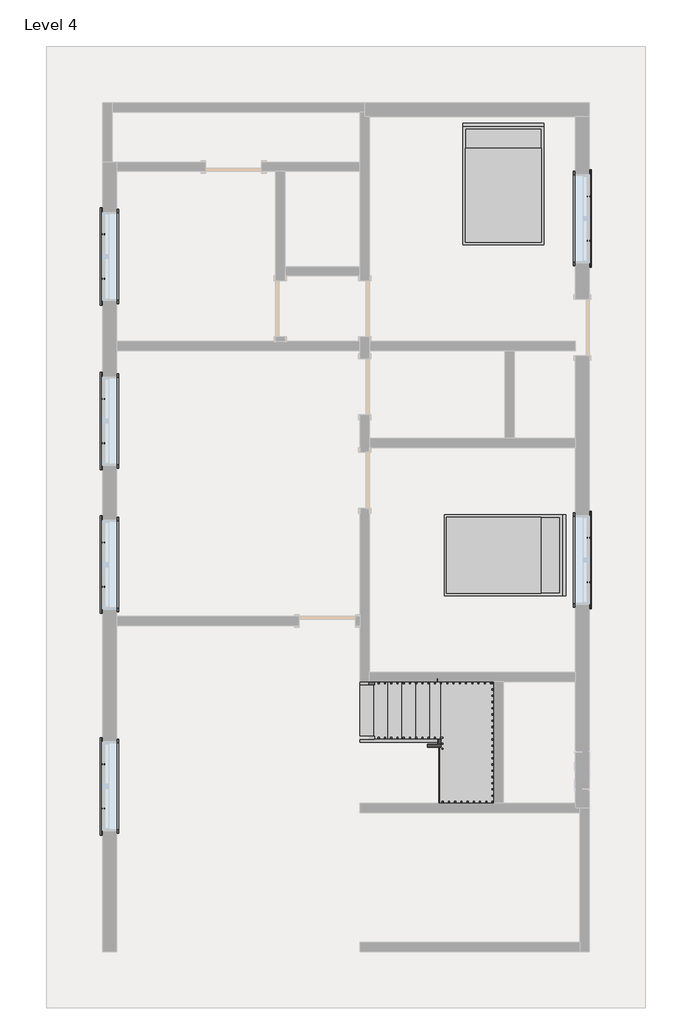
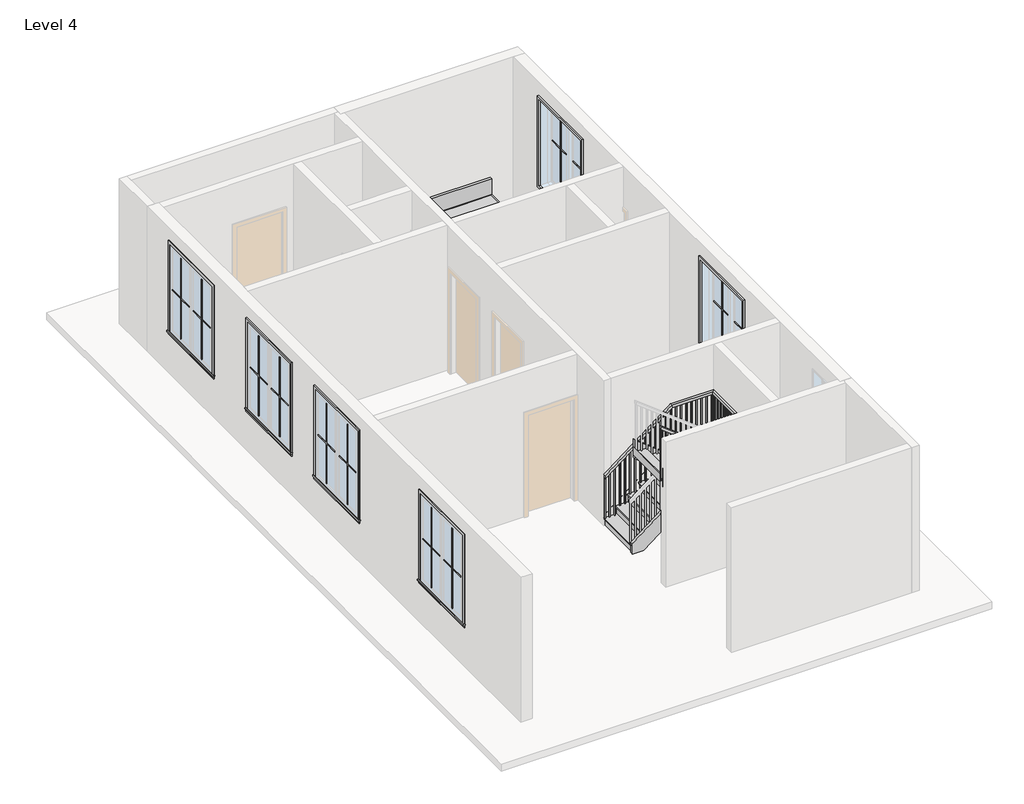
# One storey, part 2 of 2: 24 proxies, 6 members, 2 furniture elements, 1 railing, 1 stair flight.
"""IFC4 building model written with IfcOpenShell, lengths in millimetres."""

from ifc_helpers import new_model, si_unit, frame, origin, place, context, project, spatial, polyline, outline, extrude, faceted_brep, transform, mapped, element, save
from components import muntin_pattern_2x2_muntin_pattern_2x2_bff912c5, muntin_pattern_2x2_muntin_pattern_2x2_c2194282, trim_window_exterior_flat_with_sill_e04b3088, trim_window_interior_flat_picture_frame_2a7685fe, bed_17739_bed_17739_15c61121, stair_flight_6f98f22d

model = new_model("IFC4")

# Units and contexts
model_context = context("Model", 3, world=origin())
ifc_project = project(units=[si_unit("LENGTHUNIT", "METRE", prefix="MILLI")], contexts=[model_context])

# Site, building, storey
site = spatial("IfcSite", under=ifc_project)
building = spatial("IfcBuilding", under=site)
storey = spatial("IfcBuildingStorey", under=building, Name="Level 4", Elevation=6400.8)

# Proxies
placement = place(None, origin())
muntin_pattern_2x2_muntin_pattern_2x2_shape = muntin_pattern_2x2_muntin_pattern_2x2_bff912c5(model_context)
element("IfcBuildingElementProxy", 1, Name="Muntin Pattern_2x2 : Muntin Pattern_2x2", ObjectType="Muntin Pattern_2x2 : Muntin Pattern_2x2", at=placement, inside=storey, context=model_context, shape_type="MappedRepresentation", body=[
    mapped(muntin_pattern_2x2_muntin_pattern_2x2_shape, transform((-5204.1165352, 3633.8812696, 7385.05), x_axis=(0.0, 1.0, 0.0), y_axis=(-1.0, 0.0, 0.0), z_axis=(0.0, 0.0, 1.0))),
])
element("IfcBuildingElementProxy", 2, Name="Muntin Pattern_2x2 : Muntin Pattern_2x2", ObjectType="Muntin Pattern_2x2 : Muntin Pattern_2x2", at=placement, inside=storey, context=model_context, shape_type="MappedRepresentation", body=[
    mapped(muntin_pattern_2x2_muntin_pattern_2x2_shape, transform((2701.6334648, 4971.3355313, 7385.05), x_axis=(0.0, -1.0, 0.0), y_axis=(1.0, 0.0, 0.0), z_axis=(0.0, 0.0, 1.0))),
])
element("IfcBuildingElementProxy", 3, Name="Muntin Pattern_2x2 : Muntin Pattern_2x2", ObjectType="Muntin Pattern_2x2 : Muntin Pattern_2x2", at=placement, inside=storey, context=model_context, shape_type="MappedRepresentation", body=[
    mapped(muntin_pattern_2x2_muntin_pattern_2x2_shape, transform((2701.6334648, -584.9144687, 7385.05), x_axis=(0.0, -1.0, 0.0), y_axis=(1.0, 0.0, 0.0), z_axis=(0.0, 0.0, 1.0))),
])
element("IfcBuildingElementProxy", 4, Name="Muntin Pattern_2x2 : Muntin Pattern_2x2", ObjectType="Muntin Pattern_2x2 : Muntin Pattern_2x2", at=placement, inside=storey, context=model_context, shape_type="MappedRepresentation", body=[
    mapped(muntin_pattern_2x2_muntin_pattern_2x2_shape, transform((-5204.1165352, 954.9605313, 7385.05), x_axis=(0.0, 1.0, 0.0), y_axis=(-1.0, 0.0, 0.0), z_axis=(0.0, 0.0, 1.0))),
])
element("IfcBuildingElementProxy", 5, Name="Muntin Pattern_2x2 : Muntin Pattern_2x2", ObjectType="Muntin Pattern_2x2 : Muntin Pattern_2x2", at=placement, inside=storey, context=model_context, shape_type="MappedRepresentation", body=[
    mapped(muntin_pattern_2x2_muntin_pattern_2x2_shape, transform((-5204.1165352, -1381.8394687, 7385.05), x_axis=(0.0, 1.0, 0.0), y_axis=(-1.0, 0.0, 0.0), z_axis=(0.0, 0.0, 1.0))),
])
element("IfcBuildingElementProxy", 6, Name="Muntin Pattern_2x2 : Muntin Pattern_2x2", ObjectType="Muntin Pattern_2x2 : Muntin Pattern_2x2", at=placement, inside=storey, context=model_context, shape_type="MappedRepresentation", body=[
    mapped(muntin_pattern_2x2_muntin_pattern_2x2_shape, transform((-5204.1165352, -4988.6394687, 7385.05), x_axis=(0.0, 1.0, 0.0), y_axis=(-1.0, 0.0, 0.0), z_axis=(0.0, 0.0, 1.0))),
])
muntin_pattern_2x2_muntin_pattern_2x2_2_shape = muntin_pattern_2x2_muntin_pattern_2x2_c2194282(model_context)
element("IfcBuildingElementProxy", 7, Name="Muntin Pattern_2x2 : Muntin Pattern_2x2", ObjectType="Muntin Pattern_2x2 : Muntin Pattern_2x2", at=placement, inside=storey, context=model_context, shape_type="MappedRepresentation", body=[
    mapped(muntin_pattern_2x2_muntin_pattern_2x2_2_shape, transform((-5204.1165352, 4354.6062696, 7385.05), x_axis=(0.0, -1.0, 0.0), y_axis=(1.0, 0.0, 0.0), z_axis=(0.0, 0.0, 1.0))),
])
element("IfcBuildingElementProxy", 8, Name="Muntin Pattern_2x2 : Muntin Pattern_2x2", ObjectType="Muntin Pattern_2x2 : Muntin Pattern_2x2", at=placement, inside=storey, context=model_context, shape_type="MappedRepresentation", body=[
    mapped(muntin_pattern_2x2_muntin_pattern_2x2_2_shape, transform((2701.6334648, 4250.6105313, 7385.05), x_axis=(0.0, 1.0, 0.0), y_axis=(-1.0, 0.0, 0.0), z_axis=(0.0, 0.0, 1.0))),
])
element("IfcBuildingElementProxy", 9, Name="Muntin Pattern_2x2 : Muntin Pattern_2x2", ObjectType="Muntin Pattern_2x2 : Muntin Pattern_2x2", at=placement, inside=storey, context=model_context, shape_type="MappedRepresentation", body=[
    mapped(muntin_pattern_2x2_muntin_pattern_2x2_2_shape, transform((2701.6334648, -1305.6394687, 7385.05), x_axis=(0.0, 1.0, 0.0), y_axis=(-1.0, 0.0, 0.0), z_axis=(0.0, 0.0, 1.0))),
])
element("IfcBuildingElementProxy", 10, Name="Muntin Pattern_2x2 : Muntin Pattern_2x2", ObjectType="Muntin Pattern_2x2 : Muntin Pattern_2x2", at=placement, inside=storey, context=model_context, shape_type="MappedRepresentation", body=[
    mapped(muntin_pattern_2x2_muntin_pattern_2x2_2_shape, transform((-5204.1165352, 1675.6855313, 7385.05), x_axis=(0.0, -1.0, 0.0), y_axis=(1.0, 0.0, 0.0), z_axis=(0.0, 0.0, 1.0))),
])
element("IfcBuildingElementProxy", 11, Name="Muntin Pattern_2x2 : Muntin Pattern_2x2", ObjectType="Muntin Pattern_2x2 : Muntin Pattern_2x2", at=placement, inside=storey, context=model_context, shape_type="MappedRepresentation", body=[
    mapped(muntin_pattern_2x2_muntin_pattern_2x2_2_shape, transform((-5204.1165352, -661.1144687, 7385.05), x_axis=(0.0, -1.0, 0.0), y_axis=(1.0, 0.0, 0.0), z_axis=(0.0, 0.0, 1.0))),
])
element("IfcBuildingElementProxy", 12, Name="Muntin Pattern_2x2 : Muntin Pattern_2x2", ObjectType="Muntin Pattern_2x2 : Muntin Pattern_2x2", at=placement, inside=storey, context=model_context, shape_type="MappedRepresentation", body=[
    mapped(muntin_pattern_2x2_muntin_pattern_2x2_2_shape, transform((-5204.1165352, -4267.9144687, 7385.05), x_axis=(0.0, -1.0, 0.0), y_axis=(1.0, 0.0, 0.0), z_axis=(0.0, 0.0, 1.0))),
])
trim_window_exterior_flat_with_sill_shape = trim_window_exterior_flat_with_sill_e04b3088(model_context)
element("IfcBuildingElementProxy", 13, Name="Trim-Window-Exterior-Flat : with Sill", ObjectType="Trim-Window-Exterior-Flat : with Sill", at=placement, inside=storey, context=model_context, shape_type="MappedRepresentation", body=[
    mapped(trim_window_exterior_flat_with_sill_shape, transform((-5213.6415352, 3994.2437696, 9144.0), x_axis=(0.0, -1.0, 0.0), y_axis=(0.0, 0.0, 1.0), z_axis=(-1.0, 0.0, 0.0))),
])
element("IfcBuildingElementProxy", 14, Name="Trim-Window-Exterior-Flat : with Sill", ObjectType="Trim-Window-Exterior-Flat : with Sill", at=placement, inside=storey, context=model_context, shape_type="MappedRepresentation", body=[
    mapped(trim_window_exterior_flat_with_sill_shape, transform((2711.1584648, 4610.9730313, 9144.0), x_axis=(0.0, 1.0, 0.0), y_axis=(0.0, 0.0, 1.0), z_axis=(1.0, 0.0, 0.0))),
])
element("IfcBuildingElementProxy", 15, Name="Trim-Window-Exterior-Flat : with Sill", ObjectType="Trim-Window-Exterior-Flat : with Sill", at=placement, inside=storey, context=model_context, shape_type="MappedRepresentation", body=[
    mapped(trim_window_exterior_flat_with_sill_shape, transform((2711.1584648, -945.2769687, 9144.0), x_axis=(0.0, 1.0, 0.0), y_axis=(0.0, 0.0, 1.0), z_axis=(1.0, 0.0, 0.0))),
])
element("IfcBuildingElementProxy", 16, Name="Trim-Window-Exterior-Flat : with Sill", ObjectType="Trim-Window-Exterior-Flat : with Sill", at=placement, inside=storey, context=model_context, shape_type="MappedRepresentation", body=[
    mapped(trim_window_exterior_flat_with_sill_shape, transform((-5213.6415352, 1315.3230313, 9144.0), x_axis=(0.0, -1.0, 0.0), y_axis=(0.0, 0.0, 1.0), z_axis=(-1.0, 0.0, 0.0))),
])
element("IfcBuildingElementProxy", 17, Name="Trim-Window-Exterior-Flat : with Sill", ObjectType="Trim-Window-Exterior-Flat : with Sill", at=placement, inside=storey, context=model_context, shape_type="MappedRepresentation", body=[
    mapped(trim_window_exterior_flat_with_sill_shape, transform((-5213.6415352, -1021.4769687, 9144.0), x_axis=(0.0, -1.0, 0.0), y_axis=(0.0, 0.0, 1.0), z_axis=(-1.0, 0.0, 0.0))),
])
element("IfcBuildingElementProxy", 18, Name="Trim-Window-Exterior-Flat : with Sill", ObjectType="Trim-Window-Exterior-Flat : with Sill", at=placement, inside=storey, context=model_context, shape_type="MappedRepresentation", body=[
    mapped(trim_window_exterior_flat_with_sill_shape, transform((-5213.6415352, -4628.2769687, 9144.0), x_axis=(0.0, -1.0, 0.0), y_axis=(0.0, 0.0, 1.0), z_axis=(-1.0, 0.0, 0.0))),
])
trim_window_interior_flat_picture_frame_shape = trim_window_interior_flat_picture_frame_2a7685fe(model_context)
element("IfcBuildingElementProxy", 19, Name="Trim-Window-Interior-Flat : Picture Frame", ObjectType="Trim-Window-Interior-Flat : Picture Frame", at=placement, inside=storey, context=model_context, shape_type="MappedRepresentation", body=[
    mapped(trim_window_interior_flat_picture_frame_shape, transform((-4985.0415352, 3994.2437696, 9144.0), x_axis=(0.0, 1.0, 0.0), y_axis=(0.0, 0.0, 1.0), z_axis=(1.0, 0.0, 0.0))),
])
element("IfcBuildingElementProxy", 20, Name="Trim-Window-Interior-Flat : Picture Frame", ObjectType="Trim-Window-Interior-Flat : Picture Frame", at=placement, inside=storey, context=model_context, shape_type="MappedRepresentation", body=[
    mapped(trim_window_interior_flat_picture_frame_shape, transform((2482.5584648, 4610.9730313, 9144.0), x_axis=(0.0, -1.0, 0.0), y_axis=(0.0, 0.0, 1.0), z_axis=(-1.0, 0.0, 0.0))),
])
element("IfcBuildingElementProxy", 21, Name="Trim-Window-Interior-Flat : Picture Frame", ObjectType="Trim-Window-Interior-Flat : Picture Frame", at=placement, inside=storey, context=model_context, shape_type="MappedRepresentation", body=[
    mapped(trim_window_interior_flat_picture_frame_shape, transform((2482.5584648, -945.2769687, 9144.0), x_axis=(0.0, -1.0, 0.0), y_axis=(0.0, 0.0, 1.0), z_axis=(-1.0, 0.0, 0.0))),
])
element("IfcBuildingElementProxy", 22, Name="Trim-Window-Interior-Flat : Picture Frame", ObjectType="Trim-Window-Interior-Flat : Picture Frame", at=placement, inside=storey, context=model_context, shape_type="MappedRepresentation", body=[
    mapped(trim_window_interior_flat_picture_frame_shape, transform((-4985.0415352, 1315.3230313, 9144.0), x_axis=(0.0, 1.0, 0.0), y_axis=(0.0, 0.0, 1.0), z_axis=(1.0, 0.0, 0.0))),
])
element("IfcBuildingElementProxy", 23, Name="Trim-Window-Interior-Flat : Picture Frame", ObjectType="Trim-Window-Interior-Flat : Picture Frame", at=placement, inside=storey, context=model_context, shape_type="MappedRepresentation", body=[
    mapped(trim_window_interior_flat_picture_frame_shape, transform((-4985.0415352, -1021.4769687, 9144.0), x_axis=(0.0, 1.0, 0.0), y_axis=(0.0, 0.0, 1.0), z_axis=(1.0, 0.0, 0.0))),
])
element("IfcBuildingElementProxy", 24, Name="Trim-Window-Interior-Flat : Picture Frame", ObjectType="Trim-Window-Interior-Flat : Picture Frame", at=placement, inside=storey, context=model_context, shape_type="MappedRepresentation", body=[
    mapped(trim_window_interior_flat_picture_frame_shape, transform((-4985.0415352, -4628.2769687, 9144.0), x_axis=(0.0, 1.0, 0.0), y_axis=(0.0, 0.0, 1.0), z_axis=(1.0, 0.0, 0.0))),
])

# Furniture
bed_17739_bed_17739_shape = bed_17739_bed_17739_15c61121(model_context)
element("IfcFurniture", 25, ObjectType="Bed_17739 : Bed_17739", at=placement, inside=storey, context=model_context, shape_type="MappedRepresentation", body=[
    mapped(bed_17739_bed_17739_shape, transform((1314.1584648, 5149.1645078, 6400.8), x_axis=(1.0, 0.0, 0.0), y_axis=(0.0, 1.0, 0.0), z_axis=(0.0, 0.0, 1.0))),
])
element("IfcFurniture", 26, ObjectType="Bed_17739 : Bed_17739", at=placement, inside=storey, context=model_context, shape_type="MappedRepresentation", body=[
    mapped(bed_17739_bed_17739_shape, transform((1314.1584648, -869.0769687, 6400.8), x_axis=(0.0, -1.0, 0.0), y_axis=(1.0, 0.0, 0.0), z_axis=(0.0, 0.0, 1.0))),
])

# Members
element("IfcMember", 27, ObjectType="Stringer - 2\" Width", at=placement, inside=storey, context=model_context, shape_type="SweptSolid", body=[
    extrude(outline(polyline([(6622.5399812, -1022.6415352), (6400.8, -1022.6415352), (6400.8, -811.2687863), (7662.3333333, 810.8400359), (7662.3333333, 314.3488758), (6622.5399812, -1022.6415352)])), frame((0.0, -2926.4769687, 0.0), z_axis=(0.0, 1.0, 0.0), x_axis=(0.0, 0.0, 1.0)), (0.0, 0.0, 1.0), 50.8),
])
element("IfcMember", 28, ObjectType="Stringer - 2\" Width", at=placement, inside=storey, context=model_context, shape_type="SweptSolid", body=[
    extrude(outline(polyline([(1161.7584648, -2875.6769687), (1212.5584648, -2875.6769687), (1212.5584648, -4907.6769687), (1161.7584648, -4907.6769687), (1161.7584648, -2875.6769687)])), frame((0.0, 0.0, 7357.5333333), z_axis=(0.0, 0.0, 1.0), x_axis=(1.0, 0.0, 0.0)), (0.0, 0.0, 1.0), 304.8),
])
element("IfcMember", 29, ObjectType="Stringer - 2\" Width", at=placement, inside=storey, context=model_context, shape_type="SweptSolid", body=[
    extrude(outline(polyline([(7357.5333333, 884.5469698), (8840.7765283, -1022.6415352), (8454.6494451, -1022.6415352), (7357.5333333, 388.0558097), (7357.5333333, 884.5469698)])), frame((0.0, -4958.4769687, 0.0), z_axis=(0.0, 1.0, 0.0), x_axis=(0.0, 0.0, 1.0)), (0.0, 0.0, 1.0), 50.8),
])
element("IfcMember", 30, ObjectType="Stringer - 2\" Width", at=placement, inside=storey, context=model_context, shape_type="SweptSolid", body=[
    extrude(outline(polyline([(6622.5399812, -1022.6415352), (6400.8, -1022.6415352), (6400.8, -811.2687863), (7221.3567404, 243.8221038), (7607.4838236, 243.8221038), (6622.5399812, -1022.6415352)])), frame((0.0, -3912.0539367, 0.0), z_axis=(0.0, 1.0, 0.0), x_axis=(0.0, 0.0, 1.0)), (0.0, 0.0, 1.0), 50.8),
])
element("IfcMember", 31, ObjectType="Stringer - 2\" Width", at=placement, inside=storey, context=model_context, shape_type="SweptSolid", body=[
    extrude(outline(polyline([(243.8221038, -3861.2539367), (294.6221038, -3861.2539367), (294.6221038, -3942.4769687), (243.8221038, -3942.4769687), (243.8221038, -3861.2539367)])), frame((0.0, 0.0, 7357.5333333), z_axis=(0.0, 0.0, 1.0), x_axis=(1.0, 0.0, 0.0)), (0.0, 0.0, 1.0), 304.8),
])
element("IfcMember", 32, ObjectType="Stringer - 2\" Width", at=placement, inside=storey, context=model_context, shape_type="SweptSolid", body=[
    extrude(outline(polyline([(7430.1978382, 294.6221038), (7816.3249214, 294.6221038), (8840.7765283, -1022.6415352), (8454.6494451, -1022.6415352), (7430.1978382, 294.6221038)])), frame((0.0, -3993.2769687, 0.0), z_axis=(0.0, 1.0, 0.0), x_axis=(0.0, 0.0, 1.0)), (0.0, 0.0, 1.0), 50.8),
])

# Railing
element("IfcRailing", 33, ObjectType="Handrail - Rectangular", at=placement, inside=storey, context=model_context, shape_type="SolidModel", body=[
    faceted_brep([(-1022.6415352, -2926.4769687, 7484.5333333), (-1022.6415352, -2926.4769687, 7420.3783974), (-1022.6415352, -2977.2769687, 7420.3783974), (-1022.6415352, -2977.2769687, 7484.5333333), (294.6221038, -2926.4769687, 8500.5333333), (311.9370364, -2926.4769687, 8449.7333333), (311.9370364, -2977.2769687, 8449.7333333), (294.6221038, -2977.2769687, 8500.5333333), (1161.7584648, -2926.4769687, 8500.5333333), (1161.7584648, -2926.4769687, 8449.7333333), (1110.9584648, -2977.2769687, 8449.7333333), (1110.9584648, -2977.2769687, 8500.5333333), (1161.7584648, -4907.6769687, 8500.5333333), (1161.7584648, -4907.6769687, 8449.7333333), (1110.9584648, -4856.8769687, 8449.7333333), (1110.9584648, -4856.8769687, 8500.5333333), (514.1660437, -4907.6769687, 8500.5333333), (496.8511111, -4907.6769687, 8449.7333333), (496.8511111, -4856.8769687, 8449.7333333), (514.1660437, -4856.8769687, 8500.5333333), (-1022.6415352, -4907.6769687, 9685.8666667), (-1022.6415352, -4856.8769687, 9685.8666667), (-1022.6415352, -4856.8769687, 9621.7117307), (-1022.6415352, -4907.6769687, 9621.7117307)], [[[0, 1, 2, 3]], [[1, 0, 4, 5]], [[2, 1, 5, 6]], [[3, 2, 6, 7]], [[0, 3, 7, 4]], [[5, 4, 8, 9]], [[6, 5, 9, 10]], [[7, 6, 10, 11]], [[4, 7, 11, 8]], [[9, 8, 12, 13]], [[10, 9, 13, 14]], [[11, 10, 14, 15]], [[8, 11, 15, 12]], [[13, 12, 16, 17]], [[14, 13, 17, 18]], [[15, 14, 18, 19]], [[12, 15, 19, 16]], [[20, 21, 22, 23]], [[17, 16, 20, 23]], [[18, 17, 23, 22]], [[19, 18, 22, 21]], [[16, 19, 21, 20]]]),
    extrude(outline(polyline([(9609.4674089, -1006.7665352), (8602.1333333, -1006.7665352), (8602.1333333, -987.7165352), (9594.7742226, -987.7165352), (9609.4674089, -1006.7665352)])), frame((0.0, -4891.8019687, 0.0), z_axis=(0.0, 1.0, 0.0), x_axis=(0.0, 0.0, 1.0)), (0.0, 0.0, 1.0), 19.05),
    extrude(outline(polyline([(9531.1037488, -905.1665352), (8602.1333333, -905.1665352), (8602.1333333, -886.1165352), (9516.4105626, -886.1165352), (9531.1037488, -905.1665352)])), frame((0.0, -4891.8019687, 0.0), z_axis=(0.0, 1.0, 0.0), x_axis=(0.0, 0.0, 1.0)), (0.0, 0.0, 1.0), 19.05),
    extrude(outline(polyline([(9452.7400888, -803.5665352), (8602.1333333, -803.5665352), (8602.1333333, -784.5165352), (9438.0469025, -784.5165352), (9452.7400888, -803.5665352)])), frame((0.0, -4891.8019687, 0.0), z_axis=(0.0, 1.0, 0.0), x_axis=(0.0, 0.0, 1.0)), (0.0, 0.0, 1.0), 19.05),
    extrude(outline(polyline([(9374.3764287, -701.9665352), (8432.8, -701.9665352), (8432.8, -682.9165352), (9359.6832425, -682.9165352), (9374.3764287, -701.9665352)])), frame((0.0, -4891.8019687, 0.0), z_axis=(0.0, 1.0, 0.0), x_axis=(0.0, 0.0, 1.0)), (0.0, 0.0, 1.0), 19.05),
    extrude(outline(polyline([(9296.0127687, -600.3665352), (8432.8, -600.3665352), (8432.8, -581.3165352), (9281.3195824, -581.3165352), (9296.0127687, -600.3665352)])), frame((0.0, -4891.8019687, 0.0), z_axis=(0.0, 1.0, 0.0), x_axis=(0.0, 0.0, 1.0)), (0.0, 0.0, 1.0), 19.05),
    extrude(outline(polyline([(9217.6491086, -498.7665352), (8263.4666667, -498.7665352), (8263.4666667, -479.7165352), (9202.9559224, -479.7165352), (9217.6491086, -498.7665352)])), frame((0.0, -4891.8019687, 0.0), z_axis=(0.0, 1.0, 0.0), x_axis=(0.0, 0.0, 1.0)), (0.0, 0.0, 1.0), 19.05),
    extrude(outline(polyline([(9139.2854486, -397.1665352), (8263.4666667, -397.1665352), (8263.4666667, -378.1165352), (9124.5922623, -378.1165352), (9139.2854486, -397.1665352)])), frame((0.0, -4891.8019687, 0.0), z_axis=(0.0, 1.0, 0.0), x_axis=(0.0, 0.0, 1.0)), (0.0, 0.0, 1.0), 19.05),
    extrude(outline(polyline([(9060.9217885, -295.5665352), (8094.1333333, -295.5665352), (8094.1333333, -276.5165352), (9046.2286023, -276.5165352), (9060.9217885, -295.5665352)])), frame((0.0, -4891.8019687, 0.0), z_axis=(0.0, 1.0, 0.0), x_axis=(0.0, 0.0, 1.0)), (0.0, 0.0, 1.0), 19.05),
    extrude(outline(polyline([(8982.5581285, -193.9665352), (8094.1333333, -193.9665352), (8094.1333333, -174.9165352), (8967.8649422, -174.9165352), (8982.5581285, -193.9665352)])), frame((0.0, -4891.8019687, 0.0), z_axis=(0.0, 1.0, 0.0), x_axis=(0.0, 0.0, 1.0)), (0.0, 0.0, 1.0), 19.05),
    extrude(outline(polyline([(8904.1944684, -92.3665352), (7924.8, -92.3665352), (7924.8, -73.3165352), (8889.5012822, -73.3165352), (8904.1944684, -92.3665352)])), frame((0.0, -4891.8019687, 0.0), z_axis=(0.0, 1.0, 0.0), x_axis=(0.0, 0.0, 1.0)), (0.0, 0.0, 1.0), 19.05),
    extrude(outline(polyline([(8825.8308084, 9.2334648), (7924.8, 9.2334648), (7924.8, 28.2834648), (8811.1376221, 28.2834648), (8825.8308084, 9.2334648)])), frame((0.0, -4891.8019687, 0.0), z_axis=(0.0, 1.0, 0.0), x_axis=(0.0, 0.0, 1.0)), (0.0, 0.0, 1.0), 19.05),
    extrude(outline(polyline([(8747.4671484, 110.8334648), (7924.8, 110.8334648), (7924.8, 129.8834648), (8732.7739621, 129.8834648), (8747.4671484, 110.8334648)])), frame((0.0, -4891.8019687, 0.0), z_axis=(0.0, 1.0, 0.0), x_axis=(0.0, 0.0, 1.0)), (0.0, 0.0, 1.0), 19.05),
    extrude(outline(polyline([(8669.1034883, 212.4334648), (7755.4666667, 212.4334648), (7755.4666667, 231.4834648), (8654.4103021, 231.4834648), (8669.1034883, 212.4334648)])), frame((0.0, -4891.8019687, 0.0), z_axis=(0.0, 1.0, 0.0), x_axis=(0.0, 0.0, 1.0)), (0.0, 0.0, 1.0), 19.05),
    extrude(outline(polyline([(8590.7398283, 314.0334648), (7586.1333333, 314.0334648), (7586.1333333, 333.0834648), (8576.046642, 333.0834648), (8590.7398283, 314.0334648)])), frame((0.0, -4891.8019687, 0.0), z_axis=(0.0, 1.0, 0.0), x_axis=(0.0, 0.0, 1.0)), (0.0, 0.0, 1.0), 19.05),
    extrude(outline(polyline([(8512.3761682, 415.6334648), (7586.1333333, 415.6334648), (7586.1333333, 434.6834648), (8497.682982, 434.6834648), (8512.3761682, 415.6334648)])), frame((0.0, -4891.8019687, 0.0), z_axis=(0.0, 1.0, 0.0), x_axis=(0.0, 0.0, 1.0)), (0.0, 0.0, 1.0), 19.05),
    extrude(outline(polyline([(536.2834648, -4891.8019687), (517.2334648, -4891.8019687), (517.2334648, -4872.7519687), (536.2834648, -4872.7519687), (536.2834648, -4891.8019687)])), frame((0.0, 0.0, 7586.1333333), z_axis=(0.0, 0.0, 1.0), x_axis=(1.0, 0.0, 0.0)), (0.0, 0.0, 1.0), 863.6),
    extrude(outline(polyline([(637.8834648, -4891.8019687), (618.8334648, -4891.8019687), (618.8334648, -4872.7519687), (637.8834648, -4872.7519687), (637.8834648, -4891.8019687)])), frame((0.0, 0.0, 7586.1333333), z_axis=(0.0, 0.0, 1.0), x_axis=(1.0, 0.0, 0.0)), (0.0, 0.0, 1.0), 863.6),
    extrude(outline(polyline([(739.4834648, -4891.8019687), (720.4334648, -4891.8019687), (720.4334648, -4872.7519687), (739.4834648, -4872.7519687), (739.4834648, -4891.8019687)])), frame((0.0, 0.0, 7586.1333333), z_axis=(0.0, 0.0, 1.0), x_axis=(1.0, 0.0, 0.0)), (0.0, 0.0, 1.0), 863.6),
    extrude(outline(polyline([(841.0834648, -4891.8019687), (822.0334648, -4891.8019687), (822.0334648, -4872.7519687), (841.0834648, -4872.7519687), (841.0834648, -4891.8019687)])), frame((0.0, 0.0, 7586.1333333), z_axis=(0.0, 0.0, 1.0), x_axis=(1.0, 0.0, 0.0)), (0.0, 0.0, 1.0), 863.6),
    extrude(outline(polyline([(942.6834648, -4891.8019687), (923.6334648, -4891.8019687), (923.6334648, -4872.7519687), (942.6834648, -4872.7519687), (942.6834648, -4891.8019687)])), frame((0.0, 0.0, 7586.1333333), z_axis=(0.0, 0.0, 1.0), x_axis=(1.0, 0.0, 0.0)), (0.0, 0.0, 1.0), 863.6),
    extrude(outline(polyline([(1044.2834648, -4891.8019687), (1025.2334648, -4891.8019687), (1025.2334648, -4872.7519687), (1044.2834648, -4872.7519687), (1044.2834648, -4891.8019687)])), frame((0.0, 0.0, 7586.1333333), z_axis=(0.0, 0.0, 1.0), x_axis=(1.0, 0.0, 0.0)), (0.0, 0.0, 1.0), 863.6),
    extrude(outline(polyline([(1145.8834648, -4771.1519687), (1145.8834648, -4790.2019687), (1126.8334648, -4790.2019687), (1126.8334648, -4771.1519687), (1145.8834648, -4771.1519687)])), frame((0.0, 0.0, 7586.1333333), z_axis=(0.0, 0.0, 1.0), x_axis=(1.0, 0.0, 0.0)), (0.0, 0.0, 1.0), 863.6),
    extrude(outline(polyline([(1145.8834648, -4669.5519687), (1145.8834648, -4688.6019687), (1126.8334648, -4688.6019687), (1126.8334648, -4669.5519687), (1145.8834648, -4669.5519687)])), frame((0.0, 0.0, 7586.1333333), z_axis=(0.0, 0.0, 1.0), x_axis=(1.0, 0.0, 0.0)), (0.0, 0.0, 1.0), 863.6),
    extrude(outline(polyline([(1145.8834648, -4567.9519687), (1145.8834648, -4587.0019687), (1126.8334648, -4587.0019687), (1126.8334648, -4567.9519687), (1145.8834648, -4567.9519687)])), frame((0.0, 0.0, 7586.1333333), z_axis=(0.0, 0.0, 1.0), x_axis=(1.0, 0.0, 0.0)), (0.0, 0.0, 1.0), 863.6),
    extrude(outline(polyline([(1145.8834648, -4466.3519687), (1145.8834648, -4485.4019687), (1126.8334648, -4485.4019687), (1126.8334648, -4466.3519687), (1145.8834648, -4466.3519687)])), frame((0.0, 0.0, 7586.1333333), z_axis=(0.0, 0.0, 1.0), x_axis=(1.0, 0.0, 0.0)), (0.0, 0.0, 1.0), 863.6),
    extrude(outline(polyline([(1145.8834648, -4364.7519687), (1145.8834648, -4383.8019687), (1126.8334648, -4383.8019687), (1126.8334648, -4364.7519687), (1145.8834648, -4364.7519687)])), frame((0.0, 0.0, 7586.1333333), z_axis=(0.0, 0.0, 1.0), x_axis=(1.0, 0.0, 0.0)), (0.0, 0.0, 1.0), 863.6),
    extrude(outline(polyline([(1145.8834648, -4263.1519687), (1145.8834648, -4282.2019687), (1126.8334648, -4282.2019687), (1126.8334648, -4263.1519687), (1145.8834648, -4263.1519687)])), frame((0.0, 0.0, 7586.1333333), z_axis=(0.0, 0.0, 1.0), x_axis=(1.0, 0.0, 0.0)), (0.0, 0.0, 1.0), 863.6),
    extrude(outline(polyline([(1145.8834648, -4161.5519687), (1145.8834648, -4180.6019687), (1126.8334648, -4180.6019687), (1126.8334648, -4161.5519687), (1145.8834648, -4161.5519687)])), frame((0.0, 0.0, 7586.1333333), z_axis=(0.0, 0.0, 1.0), x_axis=(1.0, 0.0, 0.0)), (0.0, 0.0, 1.0), 863.6),
    extrude(outline(polyline([(1145.8834648, -4059.9519687), (1145.8834648, -4079.0019687), (1126.8334648, -4079.0019687), (1126.8334648, -4059.9519687), (1145.8834648, -4059.9519687)])), frame((0.0, 0.0, 7586.1333333), z_axis=(0.0, 0.0, 1.0), x_axis=(1.0, 0.0, 0.0)), (0.0, 0.0, 1.0), 863.6),
    extrude(outline(polyline([(1145.8834648, -3958.3519687), (1145.8834648, -3977.4019687), (1126.8334648, -3977.4019687), (1126.8334648, -3958.3519687), (1145.8834648, -3958.3519687)])), frame((0.0, 0.0, 7586.1333333), z_axis=(0.0, 0.0, 1.0), x_axis=(1.0, 0.0, 0.0)), (0.0, 0.0, 1.0), 863.6),
    extrude(outline(polyline([(1145.8834648, -3856.7519687), (1145.8834648, -3875.8019687), (1126.8334648, -3875.8019687), (1126.8334648, -3856.7519687), (1145.8834648, -3856.7519687)])), frame((0.0, 0.0, 7586.1333333), z_axis=(0.0, 0.0, 1.0), x_axis=(1.0, 0.0, 0.0)), (0.0, 0.0, 1.0), 863.6),
    extrude(outline(polyline([(1145.8834648, -3755.1519687), (1145.8834648, -3774.2019687), (1126.8334648, -3774.2019687), (1126.8334648, -3755.1519687), (1145.8834648, -3755.1519687)])), frame((0.0, 0.0, 7586.1333333), z_axis=(0.0, 0.0, 1.0), x_axis=(1.0, 0.0, 0.0)), (0.0, 0.0, 1.0), 863.6),
    extrude(outline(polyline([(1145.8834648, -3653.5519687), (1145.8834648, -3672.6019687), (1126.8334648, -3672.6019687), (1126.8334648, -3653.5519687), (1145.8834648, -3653.5519687)])), frame((0.0, 0.0, 7586.1333333), z_axis=(0.0, 0.0, 1.0), x_axis=(1.0, 0.0, 0.0)), (0.0, 0.0, 1.0), 863.6),
    extrude(outline(polyline([(1145.8834648, -3551.9519687), (1145.8834648, -3571.0019687), (1126.8334648, -3571.0019687), (1126.8334648, -3551.9519687), (1145.8834648, -3551.9519687)])), frame((0.0, 0.0, 7586.1333333), z_axis=(0.0, 0.0, 1.0), x_axis=(1.0, 0.0, 0.0)), (0.0, 0.0, 1.0), 863.6),
    extrude(outline(polyline([(1145.8834648, -3450.3519687), (1145.8834648, -3469.4019687), (1126.8334648, -3469.4019687), (1126.8334648, -3450.3519687), (1145.8834648, -3450.3519687)])), frame((0.0, 0.0, 7586.1333333), z_axis=(0.0, 0.0, 1.0), x_axis=(1.0, 0.0, 0.0)), (0.0, 0.0, 1.0), 863.6),
    extrude(outline(polyline([(1145.8834648, -3348.7519687), (1145.8834648, -3367.8019687), (1126.8334648, -3367.8019687), (1126.8334648, -3348.7519687), (1145.8834648, -3348.7519687)])), frame((0.0, 0.0, 7586.1333333), z_axis=(0.0, 0.0, 1.0), x_axis=(1.0, 0.0, 0.0)), (0.0, 0.0, 1.0), 863.6),
    extrude(outline(polyline([(1145.8834648, -3247.1519687), (1145.8834648, -3266.2019687), (1126.8334648, -3266.2019687), (1126.8334648, -3247.1519687), (1145.8834648, -3247.1519687)])), frame((0.0, 0.0, 7586.1333333), z_axis=(0.0, 0.0, 1.0), x_axis=(1.0, 0.0, 0.0)), (0.0, 0.0, 1.0), 863.6),
    extrude(outline(polyline([(1145.8834648, -3145.5519687), (1145.8834648, -3164.6019687), (1126.8334648, -3164.6019687), (1126.8334648, -3145.5519687), (1145.8834648, -3145.5519687)])), frame((0.0, 0.0, 7586.1333333), z_axis=(0.0, 0.0, 1.0), x_axis=(1.0, 0.0, 0.0)), (0.0, 0.0, 1.0), 863.6),
    extrude(outline(polyline([(1145.8834648, -3043.9519687), (1145.8834648, -3063.0019687), (1126.8334648, -3063.0019687), (1126.8334648, -3043.9519687), (1145.8834648, -3043.9519687)])), frame((0.0, 0.0, 7586.1333333), z_axis=(0.0, 0.0, 1.0), x_axis=(1.0, 0.0, 0.0)), (0.0, 0.0, 1.0), 863.6),
    extrude(outline(polyline([(1101.4334648, -2942.3519687), (1120.4834648, -2942.3519687), (1120.4834648, -2961.4019687), (1101.4334648, -2961.4019687), (1101.4334648, -2942.3519687)])), frame((0.0, 0.0, 7586.1333333), z_axis=(0.0, 0.0, 1.0), x_axis=(1.0, 0.0, 0.0)), (0.0, 0.0, 1.0), 863.6),
    extrude(outline(polyline([(999.8334648, -2942.3519687), (1018.8834648, -2942.3519687), (1018.8834648, -2961.4019687), (999.8334648, -2961.4019687), (999.8334648, -2942.3519687)])), frame((0.0, 0.0, 7586.1333333), z_axis=(0.0, 0.0, 1.0), x_axis=(1.0, 0.0, 0.0)), (0.0, 0.0, 1.0), 863.6),
    extrude(outline(polyline([(898.2334648, -2942.3519687), (917.2834648, -2942.3519687), (917.2834648, -2961.4019687), (898.2334648, -2961.4019687), (898.2334648, -2942.3519687)])), frame((0.0, 0.0, 7586.1333333), z_axis=(0.0, 0.0, 1.0), x_axis=(1.0, 0.0, 0.0)), (0.0, 0.0, 1.0), 863.6),
    extrude(outline(polyline([(796.6334648, -2942.3519687), (815.6834648, -2942.3519687), (815.6834648, -2961.4019687), (796.6334648, -2961.4019687), (796.6334648, -2942.3519687)])), frame((0.0, 0.0, 7586.1333333), z_axis=(0.0, 0.0, 1.0), x_axis=(1.0, 0.0, 0.0)), (0.0, 0.0, 1.0), 863.6),
    extrude(outline(polyline([(695.0334648, -2942.3519687), (714.0834648, -2942.3519687), (714.0834648, -2961.4019687), (695.0334648, -2961.4019687), (695.0334648, -2942.3519687)])), frame((0.0, 0.0, 7586.1333333), z_axis=(0.0, 0.0, 1.0), x_axis=(1.0, 0.0, 0.0)), (0.0, 0.0, 1.0), 863.6),
    extrude(outline(polyline([(593.4334648, -2942.3519687), (612.4834648, -2942.3519687), (612.4834648, -2961.4019687), (593.4334648, -2961.4019687), (593.4334648, -2942.3519687)])), frame((0.0, 0.0, 7586.1333333), z_axis=(0.0, 0.0, 1.0), x_axis=(1.0, 0.0, 0.0)), (0.0, 0.0, 1.0), 863.6),
    extrude(outline(polyline([(491.8334648, -2942.3519687), (510.8834648, -2942.3519687), (510.8834648, -2961.4019687), (491.8334648, -2961.4019687), (491.8334648, -2942.3519687)])), frame((0.0, 0.0, 7586.1333333), z_axis=(0.0, 0.0, 1.0), x_axis=(1.0, 0.0, 0.0)), (0.0, 0.0, 1.0), 863.6),
    extrude(outline(polyline([(390.2334648, -2942.3519687), (409.2834648, -2942.3519687), (409.2834648, -2961.4019687), (390.2334648, -2961.4019687), (390.2334648, -2942.3519687)])), frame((0.0, 0.0, 7586.1333333), z_axis=(0.0, 0.0, 1.0), x_axis=(1.0, 0.0, 0.0)), (0.0, 0.0, 1.0), 863.6),
    extrude(outline(polyline([(288.6334648, -2942.3519687), (307.6834648, -2942.3519687), (307.6834648, -2961.4019687), (288.6334648, -2961.4019687), (288.6334648, -2942.3519687)])), frame((0.0, 0.0, 7586.1333333), z_axis=(0.0, 0.0, 1.0), x_axis=(1.0, 0.0, 0.0)), (0.0, 0.0, 1.0), 863.6),
    extrude(outline(polyline([(8353.3957248, 187.0334648), (7416.8, 187.0334648), (7416.8, 206.0834648), (8368.0889111, 206.0834648), (8353.3957248, 187.0334648)])), frame((0.0, -2961.4019687, 0.0), z_axis=(0.0, 1.0, 0.0), x_axis=(0.0, 0.0, 1.0)), (0.0, 0.0, 1.0), 19.05),
    extrude(outline(polyline([(8275.0320648, 85.4334648), (7247.4666667, 85.4334648), (7247.4666667, 104.4834648), (8289.725251, 104.4834648), (8275.0320648, 85.4334648)])), frame((0.0, -2961.4019687, 0.0), z_axis=(0.0, 1.0, 0.0), x_axis=(0.0, 0.0, 1.0)), (0.0, 0.0, 1.0), 19.05),
    extrude(outline(polyline([(8196.6684047, -16.1665352), (7247.4666667, -16.1665352), (7247.4666667, 2.8834648), (8211.361591, 2.8834648), (8196.6684047, -16.1665352)])), frame((0.0, -2961.4019687, 0.0), z_axis=(0.0, 1.0, 0.0), x_axis=(0.0, 0.0, 1.0)), (0.0, 0.0, 1.0), 19.05),
    extrude(outline(polyline([(8118.3047447, -117.7665352), (7247.4666667, -117.7665352), (7247.4666667, -98.7165352), (8132.9979309, -98.7165352), (8118.3047447, -117.7665352)])), frame((0.0, -2961.4019687, 0.0), z_axis=(0.0, 1.0, 0.0), x_axis=(0.0, 0.0, 1.0)), (0.0, 0.0, 1.0), 19.05),
    extrude(outline(polyline([(8039.9410846, -219.3665352), (7078.1333333, -219.3665352), (7078.1333333, -200.3165352), (8054.6342709, -200.3165352), (8039.9410846, -219.3665352)])), frame((0.0, -2961.4019687, 0.0), z_axis=(0.0, 1.0, 0.0), x_axis=(0.0, 0.0, 1.0)), (0.0, 0.0, 1.0), 19.05),
    extrude(outline(polyline([(7961.5774246, -320.9665352), (7078.1333333, -320.9665352), (7078.1333333, -301.9165352), (7976.2706109, -301.9165352), (7961.5774246, -320.9665352)])), frame((0.0, -2961.4019687, 0.0), z_axis=(0.0, 1.0, 0.0), x_axis=(0.0, 0.0, 1.0)), (0.0, 0.0, 1.0), 19.05),
    extrude(outline(polyline([(7883.2137645, -422.5665352), (6908.8, -422.5665352), (6908.8, -403.5165352), (7897.9069508, -403.5165352), (7883.2137645, -422.5665352)])), frame((0.0, -2961.4019687, 0.0), z_axis=(0.0, 1.0, 0.0), x_axis=(0.0, 0.0, 1.0)), (0.0, 0.0, 1.0), 19.05),
    extrude(outline(polyline([(7804.8501045, -524.1665352), (6908.8, -524.1665352), (6908.8, -505.1165352), (7819.5432908, -505.1165352), (7804.8501045, -524.1665352)])), frame((0.0, -2961.4019687, 0.0), z_axis=(0.0, 1.0, 0.0), x_axis=(0.0, 0.0, 1.0)), (0.0, 0.0, 1.0), 19.05),
    extrude(outline(polyline([(7726.4864445, -625.7665352), (6739.4666667, -625.7665352), (6739.4666667, -606.7165352), (7741.1796307, -606.7165352), (7726.4864445, -625.7665352)])), frame((0.0, -2961.4019687, 0.0), z_axis=(0.0, 1.0, 0.0), x_axis=(0.0, 0.0, 1.0)), (0.0, 0.0, 1.0), 19.05),
    extrude(outline(polyline([(7648.1227844, -727.3665352), (6739.4666667, -727.3665352), (6739.4666667, -708.3165352), (7662.8159707, -708.3165352), (7648.1227844, -727.3665352)])), frame((0.0, -2961.4019687, 0.0), z_axis=(0.0, 1.0, 0.0), x_axis=(0.0, 0.0, 1.0)), (0.0, 0.0, 1.0), 19.05),
    extrude(outline(polyline([(7569.7591244, -828.9665352), (6570.1333333, -828.9665352), (6570.1333333, -809.9165352), (7584.4523106, -809.9165352), (7569.7591244, -828.9665352)])), frame((0.0, -2961.4019687, 0.0), z_axis=(0.0, 1.0, 0.0), x_axis=(0.0, 0.0, 1.0)), (0.0, 0.0, 1.0), 19.05),
    extrude(outline(polyline([(7491.3954643, -930.5665352), (6570.1333333, -930.5665352), (6570.1333333, -911.5165352), (7506.0886506, -911.5165352), (7491.3954643, -930.5665352)])), frame((0.0, -2961.4019687, 0.0), z_axis=(0.0, 1.0, 0.0), x_axis=(0.0, 0.0, 1.0)), (0.0, 0.0, 1.0), 19.05),
    extrude(outline(polyline([(1145.8834648, -4872.7519687), (1145.8834648, -4891.8019687), (1126.8334648, -4891.8019687), (1126.8334648, -4872.7519687), (1145.8834648, -4872.7519687)])), frame((0.0, 0.0, 7586.1333333), z_axis=(0.0, 0.0, 1.0), x_axis=(1.0, 0.0, 0.0)), (0.0, 0.0, 1.0), 863.6),
    extrude(outline(polyline([(1126.8334648, -2942.3519687), (1145.8834648, -2942.3519687), (1145.8834648, -2961.4019687), (1126.8334648, -2961.4019687), (1126.8334648, -2942.3519687)])), frame((0.0, 0.0, 7586.1333333), z_axis=(0.0, 0.0, 1.0), x_axis=(1.0, 0.0, 0.0)), (0.0, 0.0, 1.0), 863.6),
    extrude(outline(polyline([(9621.7117307, -1022.6415352), (8602.1333333, -1022.6415352), (8602.1333333, -1003.5915352), (9607.0185445, -1003.5915352), (9621.7117307, -1022.6415352)])), frame((0.0, -4891.8019687, 0.0), z_axis=(0.0, 1.0, 0.0), x_axis=(0.0, 0.0, 1.0)), (0.0, 0.0, 1.0), 19.05),
    extrude(outline(polyline([(7420.3783974, -1022.6415352), (6570.1333333, -1022.6415352), (6570.1333333, -1003.5915352), (7435.0715837, -1003.5915352), (7420.3783974, -1022.6415352)])), frame((0.0, -2961.4019687, 0.0), z_axis=(0.0, 1.0, 0.0), x_axis=(0.0, 0.0, 1.0)), (0.0, 0.0, 1.0), 19.05),
])

# Stair flight
stair_flight_shape = stair_flight_6f98f22d(model_context)
element("IfcStairFlight", 34, ObjectType="2\" Tread 1\" Nosing 1/4\" Riser", at=placement, inside=storey, context=model_context, shape_type="MappedRepresentation", body=[
    mapped(stair_flight_shape, transform((0.0, 0.0, 0.0), x_axis=(1.0, 0.0, 0.0), y_axis=(0.0, 1.0, 0.0), z_axis=(0.0, 0.0, 1.0))),
])

save(model, "model.ifc")

# Revit data of these elements
# Type "Muntin Pattern_2x2 : Muntin Pattern_2x2"
#   Width [instance default] = 4' - 0"
#   Thickness = 0' - 0 1/2"
#   Height [instance default] = 4' - 0"
#   Distance = 0' - 0 3/4"
#   Interior Material [instance default] = none
#   Exterior Material [instance default] = none
#   Default Elevation = 0
# Type "Trim-Window-Exterior-Flat : with Sill"
#   Trim Width = 0' - 2 1/4"
#   Trim Thickness_Picture Frame = 0' - 1 1/4"
#   Trim Thickness_with Sill = 0' - 0 3/4"
#   Sill Thickness = 0' - 1 1/4"
#   Opening Width [instance default] = 2' - 0"
#   Opening Height [instance default] = 3' - 0"
#   Default Elevation = 4' - 0"
#   Sill = yes
#   Picture Frame = no
#   Trim Material [instance default] = none
# Type "Trim-Window-Interior-Flat : Picture Frame"
#   Trim Thickness_Picture Frame = 0' - 1 1/4"
#   Trim Width = 0' - 2 1/4"
#   Trim Thickness_with Sill = 0' - 0 3/4"
#   Sill Thickness = 0' - 1 1/4"
#   Opening Width [instance default] = 2' - 0"
#   Opening Height [instance default] = 3' - 0"
#   Default Elevation = 4' - 0"
#   Sill = no
#   Picture Frame = yes
#   Trim Material [instance default] = none
# Type "Bed_17739 : Bed_17739"
#   Default Elevation = 0
# Type "Handrail - Rectangular"
#   Assembly Code = "C2010400"
#   built-in parameter 1008612 = 0.0416667 (stored number, unit not read)
#   built-in parameter 1008611 = 0.0416667 (stored number, unit not read)
#   built-in parameter 1008609 = 0.333333 (stored number, unit not read)
#   built-in parameter 1008604 = 0.166667 (stored number, unit not read)
#   built-in parameter 1008603 = 0.166667 (stored number, unit not read)
#   Railing Height = 3' - 0"
#   built-in parameter 1008630 = 2
#   built-in parameter 1008610 = 2
#   built-in parameter 1008618 = Baluster - Square : 3/4"
# Elements 1, 2, 3, 4, 5, 6, 7, 8, 9, 10, 11, 12 (IfcBuildingElementProxy, "Muntin Pattern_2x2 : Muntin Pattern_2x2")
#   Width = 1' - 11 1/8"
#   Height = 5' - 6 1/2"
#   Interior Material = Wood - Stained
#   Exterior Material = Clad - White
#   Phase Created = New Construction
#   Materials on its faces: "Clad - White", "Wood - Stained"
# Elements 13, 14, 15, 16, 17, 18 (IfcBuildingElementProxy, "Trim-Window-Exterior-Flat : with Sill")
#   Opening Width = 4' - 9"
#   Opening Height = 6' - 0"
#   Trim Material = Clad - White
#   Phase Created = New Construction
#   Materials on its faces: "Clad - White"
# Elements 19, 20, 21, 22, 23, 24 (IfcBuildingElementProxy, "Trim-Window-Interior-Flat : Picture Frame")
#   Opening Width = 4' - 9"
#   Opening Height = 6' - 0"
#   Trim Material = Wood - Stained
#   Phase Created = New Construction
#   Materials on its faces: "Wood - Stained"
# Elements 25, 26 (IfcFurniture, "Bed_17739 : Bed_17739")
#   Phase Created = New Construction
#   Materials on its faces: "legs", "sheets", "bed frame", "Blanket"
# Elements 27, 28, 29, 30, 31, 32 (IfcMember, "Stringer - 2\" Width")
#   Phase Created = New Construction
# Element 33 (IfcRailing, "Handrail - Rectangular")
#   Phase Created = New Construction
# Element 34 (IfcStairFlight, "2\" Tread 1\" Nosing 1/4\" Riser")
#   Phase Created = New Construction
# Materials
#   "Clad - White": class "Wood", colour RGB 242 242 238, transparency 0, Cost = 0
#   "Wood - Stained": class "Wood", colour RGB 224 178 126, transparency 0, Cost = 0
#   "legs": colour RGB 90 73 37, transparency 0, Cost = 0
#   "sheets": colour RGB 200 195 176, transparency 0, Cost = 0
#   "bed frame": colour RGB 90 73 37, transparency 0, Cost = 0
#   "Blanket": class "System", colour RGB 59 0 1, transparency 0, Cost = 0
